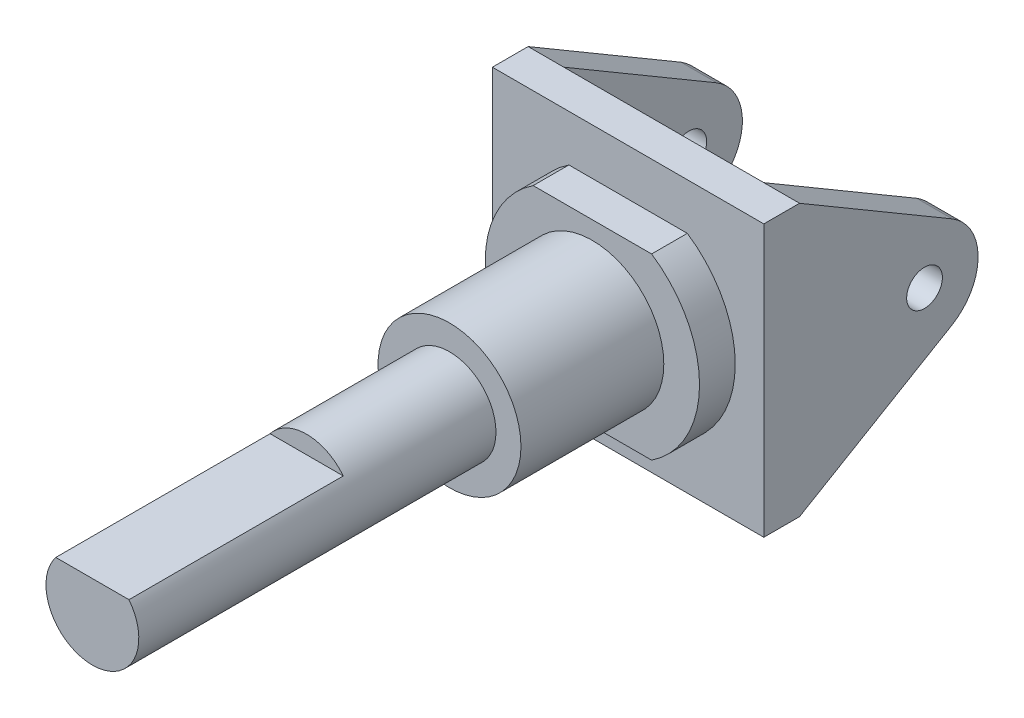
ISO-10303-21;
HEADER;
FILE_DESCRIPTION(('STEP AP214'),'2;1');
FILE_NAME('part.step','',(''),(''),'','','');
FILE_SCHEMA(('AUTOMOTIVE_DESIGN { 1 0 10303 214 1 1 1 1 }'));
ENDSEC;
DATA;
#1=APPLICATION_CONTEXT('core data for automotive mechanical design processes');
#2=APPLICATION_PROTOCOL_DEFINITION('international standard','automotive_design',2000,#1);
#3=PRODUCT_CONTEXT('',#1,'mechanical');
#4=PRODUCT('Part','Part','',(#3));
#5=PRODUCT_RELATED_PRODUCT_CATEGORY('part','',(#4));
#6=PRODUCT_DEFINITION_FORMATION('','',#4);
#7=PRODUCT_DEFINITION_CONTEXT('part definition',#1,'design');
#8=PRODUCT_DEFINITION('design','',#6,#7);
#9=PRODUCT_DEFINITION_SHAPE('','',#8);
#10=(LENGTH_UNIT() NAMED_UNIT(*) SI_UNIT(.MILLI.,.METRE.));
#11=(NAMED_UNIT(*) PLANE_ANGLE_UNIT() SI_UNIT($,.RADIAN.));
#12=(NAMED_UNIT(*) SI_UNIT($,.STERADIAN.) SOLID_ANGLE_UNIT());
#13=UNCERTAINTY_MEASURE_WITH_UNIT(LENGTH_MEASURE(1.E-05),#10,'distance_accuracy_value','');
#14=(GEOMETRIC_REPRESENTATION_CONTEXT(3) GLOBAL_UNCERTAINTY_ASSIGNED_CONTEXT((#13)) GLOBAL_UNIT_ASSIGNED_CONTEXT((#10,
#11,#12)) REPRESENTATION_CONTEXT('',''));
#15=CARTESIAN_POINT('',(0.,0.,0.));
#16=DIRECTION('',(0.,0.,1.));
#17=DIRECTION('',(1.,0.,0.));
#18=AXIS2_PLACEMENT_3D('',#15,#16,#17);
#19=CARTESIAN_POINT('',(0.,0.,20000.));
#20=DIRECTION('',(0.,0.,-1.));
#21=DIRECTION('',(-1.,0.,0.));
#22=AXIS2_PLACEMENT_3D('',#19,#20,#21);
#23=CYLINDRICAL_SURFACE('',#22,30000.);
#24=DIRECTION('',(0.,0.,-1.));
#25=VECTOR('',#24,1.);
#26=CARTESIAN_POINT('',(-16583.123951777,-25000.,20000.));
#27=LINE('',#26,#25);
#28=CARTESIAN_POINT('',(-16583.123951777,-25000.,20000.));
#29=VERTEX_POINT('',#28);
#30=CARTESIAN_POINT('',(-16583.123951777,-25000.,10000.));
#31=VERTEX_POINT('',#30);
#32=EDGE_CURVE('E194',#29,#31,#27,.T.);
#33=ORIENTED_EDGE('',*,*,#32,.F.);
#34=CARTESIAN_POINT('',(0.,0.,20000.));
#35=DIRECTION('',(0.,0.,1.));
#36=DIRECTION('',(1.,0.,0.));
#37=AXIS2_PLACEMENT_3D('',#34,#35,#36);
#38=CIRCLE('',#37,30000.);
#39=CARTESIAN_POINT('',(-16583.123951777,25000.,20000.));
#40=VERTEX_POINT('',#39);
#41=EDGE_CURVE('E197',#40,#29,#38,.T.);
#42=ORIENTED_EDGE('',*,*,#41,.F.);
#43=DIRECTION('',(0.,0.,-1.));
#44=VECTOR('',#43,1.);
#45=CARTESIAN_POINT('',(-16583.123951777,25000.,20000.));
#46=LINE('',#45,#44);
#47=CARTESIAN_POINT('',(-16583.123951777,25000.,10000.));
#48=VERTEX_POINT('',#47);
#49=EDGE_CURVE('E189',#48,#40,#46,.F.);
#50=ORIENTED_EDGE('',*,*,#49,.F.);
#51=CARTESIAN_POINT('',(0.,0.,10000.));
#52=DIRECTION('',(0.,0.,1.));
#53=DIRECTION('',(1.,0.,0.));
#54=AXIS2_PLACEMENT_3D('',#51,#52,#53);
#55=CIRCLE('',#54,30000.);
#56=EDGE_CURVE('E204',#48,#31,#55,.T.);
#57=ORIENTED_EDGE('',*,*,#56,.T.);
#58=EDGE_LOOP('',(#33,#42,#50,#57));
#59=FACE_BOUND('',#58,.T.);
#60=ADVANCED_FACE('F46',(#59),#23,.T.);
#61=DIRECTION('',(0.,0.,-1.));
#62=VECTOR('',#61,1.);
#63=CARTESIAN_POINT('',(16583.123951777,-25000.,20000.));
#64=LINE('',#63,#62);
#65=CARTESIAN_POINT('',(16583.123951777,-25000.,10000.));
#66=VERTEX_POINT('',#65);
#67=CARTESIAN_POINT('',(16583.123951777,-25000.,20000.));
#68=VERTEX_POINT('',#67);
#69=EDGE_CURVE('E68',#66,#68,#64,.F.);
#70=ORIENTED_EDGE('',*,*,#69,.F.);
#71=CARTESIAN_POINT('',(16583.123951777,25000.,10000.));
#72=VERTEX_POINT('',#71);
#73=EDGE_CURVE('E198',#66,#72,#55,.T.);
#74=ORIENTED_EDGE('',*,*,#73,.T.);
#75=DIRECTION('',(0.,0.,-1.));
#76=VECTOR('',#75,1.);
#77=CARTESIAN_POINT('',(16583.123951777,25000.,20000.));
#78=LINE('',#77,#76);
#79=CARTESIAN_POINT('',(16583.123951777,25000.,20000.));
#80=VERTEX_POINT('',#79);
#81=EDGE_CURVE('E188',#80,#72,#78,.T.);
#82=ORIENTED_EDGE('',*,*,#81,.F.);
#83=EDGE_CURVE('E193',#68,#80,#38,.T.);
#84=ORIENTED_EDGE('',*,*,#83,.F.);
#85=EDGE_LOOP('',(#70,#74,#82,#84));
#86=FACE_BOUND('',#85,.T.);
#87=ADVANCED_FACE('F304',(#86),#23,.T.);
#88=CARTESIAN_POINT('',(0.,0.,20000.));
#89=DIRECTION('',(0.,0.,1.));
#90=DIRECTION('',(1.,0.,0.));
#91=AXIS2_PLACEMENT_3D('',#88,#89,#90);
#92=PLANE('',#91);
#93=CARTESIAN_POINT('',(0.,0.,20000.));
#94=DIRECTION('',(0.,0.,1.));
#95=DIRECTION('',(1.,0.,0.));
#96=AXIS2_PLACEMENT_3D('',#93,#94,#95);
#97=CIRCLE('',#96,20000.);
#98=CARTESIAN_POINT('',(20000.,0.,20000.));
#99=VERTEX_POINT('',#98);
#100=EDGE_CURVE('E179',#99,#99,#97,.T.);
#101=ORIENTED_EDGE('',*,*,#100,.F.);
#102=EDGE_LOOP('',(#101));
#103=FACE_BOUND('',#102,.T.);
#104=ORIENTED_EDGE('',*,*,#41,.T.);
#105=DIRECTION('',(1.,0.,0.));
#106=VECTOR('',#105,1.);
#107=CARTESIAN_POINT('',(0.,-25000.,20000.));
#108=LINE('',#107,#106);
#109=EDGE_CURVE('E183',#29,#68,#108,.T.);
#110=ORIENTED_EDGE('',*,*,#109,.T.);
#111=ORIENTED_EDGE('',*,*,#83,.T.);
#112=DIRECTION('',(-1.,0.,0.));
#113=VECTOR('',#112,1.);
#114=CARTESIAN_POINT('',(0.,25000.,20000.));
#115=LINE('',#114,#113);
#116=EDGE_CURVE('E295',#80,#40,#115,.T.);
#117=ORIENTED_EDGE('',*,*,#116,.T.);
#118=EDGE_LOOP('',(#104,#110,#111,#117));
#119=FACE_BOUND('',#118,.T.);
#120=ADVANCED_FACE('F297',(#103,#119),#92,.T.);
#121=CARTESIAN_POINT('',(0.,0.,0.));
#122=DIRECTION('',(0.,0.,-1.));
#123=DIRECTION('',(-1.,0.,0.));
#124=AXIS2_PLACEMENT_3D('',#121,#122,#123);
#125=PLANE('',#124);
#126=DIRECTION('',(1.,0.,0.));
#127=VECTOR('',#126,1.);
#128=CARTESIAN_POINT('',(-38000.,-38000.,0.));
#129=LINE('',#128,#127);
#130=CARTESIAN_POINT('',(-28000.,-38000.,0.));
#131=VERTEX_POINT('',#130);
#132=CARTESIAN_POINT('',(28000.,-38000.,0.));
#133=VERTEX_POINT('',#132);
#134=EDGE_CURVE('E285',#131,#133,#129,.T.);
#135=ORIENTED_EDGE('',*,*,#134,.F.);
#136=DIRECTION('',(0.,1.,0.));
#137=VECTOR('',#136,1.);
#138=CARTESIAN_POINT('',(-28000.,38000.,0.));
#139=LINE('',#138,#137);
#140=CARTESIAN_POINT('',(-28000.,38000.,0.));
#141=VERTEX_POINT('',#140);
#142=EDGE_CURVE('E219',#131,#141,#139,.T.);
#143=ORIENTED_EDGE('',*,*,#142,.T.);
#144=DIRECTION('',(-1.,0.,0.));
#145=VECTOR('',#144,1.);
#146=CARTESIAN_POINT('',(-38000.,38000.,0.));
#147=LINE('',#146,#145);
#148=CARTESIAN_POINT('',(28000.,38000.,0.));
#149=VERTEX_POINT('',#148);
#150=EDGE_CURVE('E264',#149,#141,#147,.T.);
#151=ORIENTED_EDGE('',*,*,#150,.F.);
#152=DIRECTION('',(0.,1.,0.));
#153=VECTOR('',#152,1.);
#154=CARTESIAN_POINT('',(28000.,0.,0.));
#155=LINE('',#154,#153);
#156=EDGE_CURVE('E248',#133,#149,#155,.T.);
#157=ORIENTED_EDGE('',*,*,#156,.F.);
#158=EDGE_LOOP('',(#135,#143,#151,#157));
#159=FACE_BOUND('',#158,.T.);
#160=ADVANCED_FACE('F385',(#159),#125,.T.);
#161=CARTESIAN_POINT('',(38000.,-38000.,10000.));
#162=DIRECTION('',(-1.,0.,0.));
#163=DIRECTION('',(0.,0.,1.));
#164=AXIS2_PLACEMENT_3D('',#161,#162,#163);
#165=PLANE('',#164);
#166=DIRECTION('',(0.,0.,-1.));
#167=VECTOR('',#166,1.);
#168=CARTESIAN_POINT('',(38000.,-38000.,10000.));
#169=LINE('',#168,#167);
#170=CARTESIAN_POINT('',(38000.,-38000.,10000.));
#171=VERTEX_POINT('',#170);
#172=CARTESIAN_POINT('',(38000.,-38000.,0.));
#173=VERTEX_POINT('',#172);
#174=EDGE_CURVE('E276',#171,#173,#169,.T.);
#175=ORIENTED_EDGE('',*,*,#174,.T.);
#176=DIRECTION('',(0.,0.507188321377975,-0.861835254940172));
#177=VECTOR('',#176,1.);
#178=CARTESIAN_POINT('',(38000.,-28224.8802529961,-16610.2854977837));
#179=LINE('',#178,#177);
#180=CARTESIAN_POINT('',(38000.,-12806.4007433783,-42810.));
#181=VERTEX_POINT('',#180);
#182=EDGE_CURVE('E253',#173,#181,#179,.T.);
#183=ORIENTED_EDGE('',*,*,#182,.T.);
#184=CARTESIAN_POINT('',(38000.,0.,-35000.));
#185=DIRECTION('',(1.,0.,0.));
#186=DIRECTION('',(0.,0.,-1.));
#187=AXIS2_PLACEMENT_3D('',#184,#185,#186);
#188=CIRCLE('',#187,15000.);
#189=CARTESIAN_POINT('',(38000.,12807.4778876911,-42808.2334850018));
#190=VERTEX_POINT('',#189);
#191=EDGE_CURVE('E259',#181,#190,#188,.T.);
#192=ORIENTED_EDGE('',*,*,#191,.T.);
#193=DIRECTION('',(0.,-0.507187759813916,-0.86183558541925));
#194=VECTOR('',#193,1.);
#195=CARTESIAN_POINT('',(38000.,28224.9018992078,-16610.2734760748));
#196=LINE('',#195,#194);
#197=CARTESIAN_POINT('',(38000.,38000.,0.));
#198=VERTEX_POINT('',#197);
#199=EDGE_CURVE('E241',#198,#190,#196,.T.);
#200=ORIENTED_EDGE('',*,*,#199,.F.);
#201=DIRECTION('',(0.,0.,-1.));
#202=VECTOR('',#201,1.);
#203=CARTESIAN_POINT('',(38000.,38000.,10000.));
#204=LINE('',#203,#202);
#205=CARTESIAN_POINT('',(38000.,38000.,10000.));
#206=VERTEX_POINT('',#205);
#207=EDGE_CURVE('E202',#206,#198,#204,.T.);
#208=ORIENTED_EDGE('',*,*,#207,.F.);
#209=DIRECTION('',(0.,1.,0.));
#210=VECTOR('',#209,1.);
#211=CARTESIAN_POINT('',(38000.,-38000.,10000.));
#212=LINE('',#211,#210);
#213=EDGE_CURVE('E270',#171,#206,#212,.T.);
#214=ORIENTED_EDGE('',*,*,#213,.F.);
#215=EDGE_LOOP('',(#175,#183,#192,#200,#208,#214));
#216=FACE_BOUND('',#215,.T.);
#217=CARTESIAN_POINT('',(38000.,0.,-35000.));
#218=DIRECTION('',(1.,0.,0.));
#219=DIRECTION('',(0.,0.,-1.));
#220=AXIS2_PLACEMENT_3D('',#217,#218,#219);
#221=CIRCLE('',#220,5000.);
#222=CARTESIAN_POINT('',(38000.,0.,-40000.));
#223=VERTEX_POINT('',#222);
#224=EDGE_CURVE('E231',#223,#223,#221,.T.);
#225=ORIENTED_EDGE('',*,*,#224,.F.);
#226=EDGE_LOOP('',(#225));
#227=FACE_BOUND('',#226,.T.);
#228=ADVANCED_FACE('F48',(#216,#227),#165,.F.);
#229=CARTESIAN_POINT('',(-38000.,38000.,10000.));
#230=DIRECTION('',(0.,-1.,0.));
#231=DIRECTION('',(0.,0.,-1.));
#232=AXIS2_PLACEMENT_3D('',#229,#230,#231);
#233=PLANE('',#232);
#234=EDGE_CURVE('E278',#198,#149,#147,.T.);
#235=ORIENTED_EDGE('',*,*,#234,.T.);
#236=ORIENTED_EDGE('',*,*,#150,.T.);
#237=DIRECTION('',(-1.,0.,0.));
#238=VECTOR('',#237,1.);
#239=CARTESIAN_POINT('',(-28000.,38000.,0.));
#240=LINE('',#239,#238);
#241=CARTESIAN_POINT('',(-38000.,38000.,0.));
#242=VERTEX_POINT('',#241);
#243=EDGE_CURVE('E229',#141,#242,#240,.T.);
#244=ORIENTED_EDGE('',*,*,#243,.T.);
#245=DIRECTION('',(0.,0.,-1.));
#246=VECTOR('',#245,1.);
#247=CARTESIAN_POINT('',(-38000.,38000.,10000.));
#248=LINE('',#247,#246);
#249=CARTESIAN_POINT('',(-38000.,38000.,10000.));
#250=VERTEX_POINT('',#249);
#251=EDGE_CURVE('E286',#250,#242,#248,.T.);
#252=ORIENTED_EDGE('',*,*,#251,.F.);
#253=DIRECTION('',(-1.,0.,0.));
#254=VECTOR('',#253,1.);
#255=CARTESIAN_POINT('',(-38000.,38000.,10000.));
#256=LINE('',#255,#254);
#257=EDGE_CURVE('E275',#206,#250,#256,.T.);
#258=ORIENTED_EDGE('',*,*,#257,.F.);
#259=ORIENTED_EDGE('',*,*,#207,.T.);
#260=EDGE_LOOP('',(#235,#236,#244,#252,#258,#259));
#261=FACE_BOUND('',#260,.T.);
#262=ADVANCED_FACE('F391',(#261),#233,.F.);
#263=CARTESIAN_POINT('',(-38000.,-38000.,10000.));
#264=DIRECTION('',(1.,0.,0.));
#265=DIRECTION('',(0.,0.,-1.));
#266=AXIS2_PLACEMENT_3D('',#263,#264,#265);
#267=PLANE('',#266);
#268=ORIENTED_EDGE('',*,*,#251,.T.);
#269=DIRECTION('',(0.,-0.507198614788399,-0.861829197205994));
#270=VECTOR('',#269,1.);
#271=CARTESIAN_POINT('',(-38000.,38000.,0.));
#272=LINE('',#271,#270);
#273=CARTESIAN_POINT('',(-38000.,12788.0569282436,-42840.));
#274=VERTEX_POINT('',#273);
#275=EDGE_CURVE('E210',#242,#274,#272,.T.);
#276=ORIENTED_EDGE('',*,*,#275,.T.);
#277=CARTESIAN_POINT('',(-38000.,0.,-35000.));
#278=DIRECTION('',(-1.,0.,0.));
#279=DIRECTION('',(0.,0.,1.));
#280=AXIS2_PLACEMENT_3D('',#277,#278,#279);
#281=CIRCLE('',#280,15000.);
#282=CARTESIAN_POINT('',(-38000.,-12788.0569282436,-42840.));
#283=VERTEX_POINT('',#282);
#284=EDGE_CURVE('E228',#274,#283,#281,.T.);
#285=ORIENTED_EDGE('',*,*,#284,.T.);
#286=DIRECTION('',(0.,-0.507198614788399,0.861829197205994));
#287=VECTOR('',#286,1.);
#288=CARTESIAN_POINT('',(-38000.,-38000.,0.));
#289=LINE('',#288,#287);
#290=CARTESIAN_POINT('',(-38000.,-38000.,0.));
#291=VERTEX_POINT('',#290);
#292=EDGE_CURVE('E213',#283,#291,#289,.T.);
#293=ORIENTED_EDGE('',*,*,#292,.T.);
#294=DIRECTION('',(0.,0.,-1.));
#295=VECTOR('',#294,1.);
#296=CARTESIAN_POINT('',(-38000.,-38000.,10000.));
#297=LINE('',#296,#295);
#298=CARTESIAN_POINT('',(-38000.,-38000.,10000.));
#299=VERTEX_POINT('',#298);
#300=EDGE_CURVE('E289',#299,#291,#297,.T.);
#301=ORIENTED_EDGE('',*,*,#300,.F.);
#302=DIRECTION('',(0.,-1.,0.));
#303=VECTOR('',#302,1.);
#304=CARTESIAN_POINT('',(-38000.,-38000.,10000.));
#305=LINE('',#304,#303);
#306=EDGE_CURVE('E273',#250,#299,#305,.T.);
#307=ORIENTED_EDGE('',*,*,#306,.F.);
#308=EDGE_LOOP('',(#268,#276,#285,#293,#301,#307));
#309=FACE_BOUND('',#308,.T.);
#310=CARTESIAN_POINT('',(-38000.,0.,-35000.));
#311=DIRECTION('',(-1.,0.,0.));
#312=DIRECTION('',(0.,0.,1.));
#313=AXIS2_PLACEMENT_3D('',#310,#311,#312);
#314=CIRCLE('',#313,5000.);
#315=CARTESIAN_POINT('',(-38000.,0.,-30000.));
#316=VERTEX_POINT('',#315);
#317=EDGE_CURVE('E206',#316,#316,#314,.T.);
#318=ORIENTED_EDGE('',*,*,#317,.F.);
#319=EDGE_LOOP('',(#318));
#320=FACE_BOUND('',#319,.T.);
#321=ADVANCED_FACE('F389',(#309,#320),#267,.F.);
#322=CARTESIAN_POINT('',(-38000.,-38000.,10000.));
#323=DIRECTION('',(0.,1.,0.));
#324=DIRECTION('',(0.,0.,1.));
#325=AXIS2_PLACEMENT_3D('',#322,#323,#324);
#326=PLANE('',#325);
#327=EDGE_CURVE('E271',#291,#131,#129,.T.);
#328=ORIENTED_EDGE('',*,*,#327,.T.);
#329=ORIENTED_EDGE('',*,*,#134,.T.);
#330=DIRECTION('',(1.,0.,0.));
#331=VECTOR('',#330,1.);
#332=CARTESIAN_POINT('',(28000.,-38000.,0.));
#333=LINE('',#332,#331);
#334=EDGE_CURVE('E262',#133,#173,#333,.T.);
#335=ORIENTED_EDGE('',*,*,#334,.T.);
#336=ORIENTED_EDGE('',*,*,#174,.F.);
#337=DIRECTION('',(1.,0.,0.));
#338=VECTOR('',#337,1.);
#339=CARTESIAN_POINT('',(-38000.,-38000.,10000.));
#340=LINE('',#339,#338);
#341=EDGE_CURVE('E280',#299,#171,#340,.T.);
#342=ORIENTED_EDGE('',*,*,#341,.F.);
#343=ORIENTED_EDGE('',*,*,#300,.T.);
#344=EDGE_LOOP('',(#328,#329,#335,#336,#342,#343));
#345=FACE_BOUND('',#344,.T.);
#346=ADVANCED_FACE('F382',(#345),#326,.F.);
#347=CARTESIAN_POINT('',(0.,0.,10000.));
#348=DIRECTION('',(0.,0.,-1.));
#349=DIRECTION('',(-1.,0.,0.));
#350=AXIS2_PLACEMENT_3D('',#347,#348,#349);
#351=PLANE('',#350);
#352=ORIENTED_EDGE('',*,*,#73,.F.);
#353=DIRECTION('',(1.,0.,0.));
#354=VECTOR('',#353,1.);
#355=CARTESIAN_POINT('',(-35000.,-25000.,10000.));
#356=LINE('',#355,#354);
#357=EDGE_CURVE('E187',#31,#66,#356,.T.);
#358=ORIENTED_EDGE('',*,*,#357,.F.);
#359=ORIENTED_EDGE('',*,*,#56,.F.);
#360=DIRECTION('',(-1.,0.,0.));
#361=VECTOR('',#360,1.);
#362=CARTESIAN_POINT('',(-35000.,25000.,10000.));
#363=LINE('',#362,#361);
#364=EDGE_CURVE('E174',#72,#48,#363,.T.);
#365=ORIENTED_EDGE('',*,*,#364,.F.);
#366=EDGE_LOOP('',(#352,#358,#359,#365));
#367=FACE_BOUND('',#366,.T.);
#368=ORIENTED_EDGE('',*,*,#213,.T.);
#369=ORIENTED_EDGE('',*,*,#257,.T.);
#370=ORIENTED_EDGE('',*,*,#306,.T.);
#371=ORIENTED_EDGE('',*,*,#341,.T.);
#372=EDGE_LOOP('',(#368,#369,#370,#371));
#373=FACE_BOUND('',#372,.T.);
#374=ADVANCED_FACE('F312',(#367,#373),#351,.F.);
#375=CARTESIAN_POINT('',(28000.,-28224.8802529961,-16610.2854977837));
#376=DIRECTION('',(0.,-0.861835254940172,-0.507188321377975));
#377=DIRECTION('',(0.,0.507188321377975,-0.861835254940172));
#378=AXIS2_PLACEMENT_3D('',#375,#376,#377);
#379=PLANE('',#378);
#380=ORIENTED_EDGE('',*,*,#182,.F.);
#381=ORIENTED_EDGE('',*,*,#334,.F.);
#382=DIRECTION('',(0.,0.507188321377975,-0.861835254940172));
#383=VECTOR('',#382,1.);
#384=CARTESIAN_POINT('',(28000.,-28224.8802529961,-16610.2854977837));
#385=LINE('',#384,#383);
#386=CARTESIAN_POINT('',(28000.,-12806.4007433783,-42810.));
#387=VERTEX_POINT('',#386);
#388=EDGE_CURVE('E239',#133,#387,#385,.T.);
#389=ORIENTED_EDGE('',*,*,#388,.T.);
#390=DIRECTION('',(1.,0.,0.));
#391=VECTOR('',#390,1.);
#392=CARTESIAN_POINT('',(28000.,-12806.4007433783,-42810.));
#393=LINE('',#392,#391);
#394=EDGE_CURVE('E255',#387,#181,#393,.T.);
#395=ORIENTED_EDGE('',*,*,#394,.T.);
#396=EDGE_LOOP('',(#380,#381,#389,#395));
#397=FACE_BOUND('',#396,.T.);
#398=ADVANCED_FACE('F368',(#397),#379,.T.);
#399=CARTESIAN_POINT('',(28000.,28224.9018992078,-16610.2734760748));
#400=DIRECTION('',(0.,-0.86183558541925,0.507187759813916));
#401=DIRECTION('',(0.,-0.507187759813916,-0.86183558541925));
#402=AXIS2_PLACEMENT_3D('',#399,#400,#401);
#403=PLANE('',#402);
#404=ORIENTED_EDGE('',*,*,#199,.T.);
#405=DIRECTION('',(1.,0.,0.));
#406=VECTOR('',#405,1.);
#407=CARTESIAN_POINT('',(28000.,12807.4778876911,-42808.2334850018));
#408=LINE('',#407,#406);
#409=CARTESIAN_POINT('',(28000.,12807.4778876911,-42808.2334850018));
#410=VERTEX_POINT('',#409);
#411=EDGE_CURVE('E268',#410,#190,#408,.T.);
#412=ORIENTED_EDGE('',*,*,#411,.F.);
#413=DIRECTION('',(0.,-0.507187759813916,-0.86183558541925));
#414=VECTOR('',#413,1.);
#415=CARTESIAN_POINT('',(28000.,28224.9018992078,-16610.2734760748));
#416=LINE('',#415,#414);
#417=EDGE_CURVE('E250',#149,#410,#416,.T.);
#418=ORIENTED_EDGE('',*,*,#417,.F.);
#419=ORIENTED_EDGE('',*,*,#234,.F.);
#420=EDGE_LOOP('',(#404,#412,#418,#419));
#421=FACE_BOUND('',#420,.T.);
#422=ADVANCED_FACE('F364',(#421),#403,.F.);
#423=CARTESIAN_POINT('',(28000.,0.,-35000.));
#424=DIRECTION('',(1.,0.,0.));
#425=DIRECTION('',(0.,0.,-1.));
#426=AXIS2_PLACEMENT_3D('',#423,#424,#425);
#427=CYLINDRICAL_SURFACE('',#426,5000.);
#428=CARTESIAN_POINT('',(28000.,0.,-35000.));
#429=DIRECTION('',(1.,0.,0.));
#430=DIRECTION('',(0.,0.,-1.));
#431=AXIS2_PLACEMENT_3D('',#428,#429,#430);
#432=CIRCLE('',#431,5000.);
#433=CARTESIAN_POINT('',(28000.,0.,-40000.));
#434=VERTEX_POINT('',#433);
#435=EDGE_CURVE('E240',#434,#434,#432,.T.);
#436=ORIENTED_EDGE('',*,*,#435,.F.);
#437=EDGE_LOOP('',(#436));
#438=FACE_BOUND('',#437,.T.);
#439=ORIENTED_EDGE('',*,*,#224,.T.);
#440=EDGE_LOOP('',(#439));
#441=FACE_BOUND('',#440,.T.);
#442=ADVANCED_FACE('F370',(#438,#441),#427,.F.);
#443=CARTESIAN_POINT('',(28000.,0.,-35000.));
#444=DIRECTION('',(1.,0.,0.));
#445=DIRECTION('',(0.,0.,-1.));
#446=AXIS2_PLACEMENT_3D('',#443,#444,#445);
#447=CYLINDRICAL_SURFACE('',#446,15000.);
#448=ORIENTED_EDGE('',*,*,#191,.F.);
#449=ORIENTED_EDGE('',*,*,#394,.F.);
#450=CARTESIAN_POINT('',(28000.,0.,-35000.));
#451=DIRECTION('',(1.,0.,0.));
#452=DIRECTION('',(0.,0.,-1.));
#453=AXIS2_PLACEMENT_3D('',#450,#451,#452);
#454=CIRCLE('',#453,15000.);
#455=EDGE_CURVE('E242',#387,#410,#454,.T.);
#456=ORIENTED_EDGE('',*,*,#455,.T.);
#457=ORIENTED_EDGE('',*,*,#411,.T.);
#458=EDGE_LOOP('',(#448,#449,#456,#457));
#459=FACE_BOUND('',#458,.T.);
#460=ADVANCED_FACE('F365',(#459),#447,.T.);
#461=CARTESIAN_POINT('',(28000.,0.,0.));
#462=DIRECTION('',(1.,0.,0.));
#463=DIRECTION('',(0.,0.,-1.));
#464=AXIS2_PLACEMENT_3D('',#461,#462,#463);
#465=PLANE('',#464);
#466=ORIENTED_EDGE('',*,*,#435,.T.);
#467=EDGE_LOOP('',(#466));
#468=FACE_BOUND('',#467,.T.);
#469=ORIENTED_EDGE('',*,*,#388,.F.);
#470=ORIENTED_EDGE('',*,*,#156,.T.);
#471=ORIENTED_EDGE('',*,*,#417,.T.);
#472=ORIENTED_EDGE('',*,*,#455,.F.);
#473=EDGE_LOOP('',(#469,#470,#471,#472));
#474=FACE_BOUND('',#473,.T.);
#475=ADVANCED_FACE('F356',(#468,#474),#465,.F.);
#476=CARTESIAN_POINT('',(-28000.,38000.,0.));
#477=DIRECTION('',(0.,0.861829197205995,-0.507198614788399));
#478=DIRECTION('',(0.,0.507198614788399,0.861829197205995));
#479=AXIS2_PLACEMENT_3D('',#476,#477,#478);
#480=PLANE('',#479);
#481=ORIENTED_EDGE('',*,*,#275,.F.);
#482=ORIENTED_EDGE('',*,*,#243,.F.);
#483=DIRECTION('',(0.,-0.507198614788399,-0.861829197205994));
#484=VECTOR('',#483,1.);
#485=CARTESIAN_POINT('',(-28000.,38000.,0.));
#486=LINE('',#485,#484);
#487=CARTESIAN_POINT('',(-28000.,12788.0569282436,-42840.));
#488=VERTEX_POINT('',#487);
#489=EDGE_CURVE('E212',#141,#488,#486,.T.);
#490=ORIENTED_EDGE('',*,*,#489,.T.);
#491=DIRECTION('',(-1.,0.,0.));
#492=VECTOR('',#491,1.);
#493=CARTESIAN_POINT('',(-28000.,12788.0569282436,-42840.));
#494=LINE('',#493,#492);
#495=EDGE_CURVE('E222',#488,#274,#494,.T.);
#496=ORIENTED_EDGE('',*,*,#495,.T.);
#497=EDGE_LOOP('',(#481,#482,#490,#496));
#498=FACE_BOUND('',#497,.T.);
#499=ADVANCED_FACE('F353',(#498),#480,.T.);
#500=CARTESIAN_POINT('',(-28000.,-38000.,0.));
#501=DIRECTION('',(0.,-0.861829197205995,-0.507198614788399));
#502=DIRECTION('',(0.,0.507198614788399,-0.861829197205995));
#503=AXIS2_PLACEMENT_3D('',#500,#501,#502);
#504=PLANE('',#503);
#505=ORIENTED_EDGE('',*,*,#292,.F.);
#506=DIRECTION('',(-1.,0.,0.));
#507=VECTOR('',#506,1.);
#508=CARTESIAN_POINT('',(-28000.,-12788.0569282436,-42840.));
#509=LINE('',#508,#507);
#510=CARTESIAN_POINT('',(-28000.,-12788.0569282436,-42840.));
#511=VERTEX_POINT('',#510);
#512=EDGE_CURVE('E234',#511,#283,#509,.T.);
#513=ORIENTED_EDGE('',*,*,#512,.F.);
#514=DIRECTION('',(0.,-0.507198614788399,0.861829197205994));
#515=VECTOR('',#514,1.);
#516=CARTESIAN_POINT('',(-28000.,-38000.,0.));
#517=LINE('',#516,#515);
#518=EDGE_CURVE('E217',#511,#131,#517,.T.);
#519=ORIENTED_EDGE('',*,*,#518,.T.);
#520=ORIENTED_EDGE('',*,*,#327,.F.);
#521=EDGE_LOOP('',(#505,#513,#519,#520));
#522=FACE_BOUND('',#521,.T.);
#523=ADVANCED_FACE('F347',(#522),#504,.T.);
#524=CARTESIAN_POINT('',(-28000.,0.,-35000.));
#525=DIRECTION('',(-1.,0.,0.));
#526=DIRECTION('',(0.,0.,1.));
#527=AXIS2_PLACEMENT_3D('',#524,#525,#526);
#528=CYLINDRICAL_SURFACE('',#527,15000.);
#529=ORIENTED_EDGE('',*,*,#284,.F.);
#530=ORIENTED_EDGE('',*,*,#495,.F.);
#531=CARTESIAN_POINT('',(-28000.,0.,-35000.));
#532=DIRECTION('',(-1.,0.,0.));
#533=DIRECTION('',(0.,0.,1.));
#534=AXIS2_PLACEMENT_3D('',#531,#532,#533);
#535=CIRCLE('',#534,15000.);
#536=EDGE_CURVE('E211',#488,#511,#535,.T.);
#537=ORIENTED_EDGE('',*,*,#536,.T.);
#538=ORIENTED_EDGE('',*,*,#512,.T.);
#539=EDGE_LOOP('',(#529,#530,#537,#538));
#540=FACE_BOUND('',#539,.T.);
#541=ADVANCED_FACE('F346',(#540),#528,.T.);
#542=CARTESIAN_POINT('',(-28000.,0.,-35000.));
#543=DIRECTION('',(-1.,0.,0.));
#544=DIRECTION('',(0.,0.,1.));
#545=AXIS2_PLACEMENT_3D('',#542,#543,#544);
#546=PLANE('',#545);
#547=CARTESIAN_POINT('',(-28000.,0.,-35000.));
#548=DIRECTION('',(-1.,0.,0.));
#549=DIRECTION('',(0.,0.,1.));
#550=AXIS2_PLACEMENT_3D('',#547,#548,#549);
#551=CIRCLE('',#550,5000.);
#552=CARTESIAN_POINT('',(-28000.,0.,-30000.));
#553=VERTEX_POINT('',#552);
#554=EDGE_CURVE('E205',#553,#553,#551,.T.);
#555=ORIENTED_EDGE('',*,*,#554,.T.);
#556=EDGE_LOOP('',(#555));
#557=FACE_BOUND('',#556,.T.);
#558=ORIENTED_EDGE('',*,*,#489,.F.);
#559=ORIENTED_EDGE('',*,*,#142,.F.);
#560=ORIENTED_EDGE('',*,*,#518,.F.);
#561=ORIENTED_EDGE('',*,*,#536,.F.);
#562=EDGE_LOOP('',(#558,#559,#560,#561));
#563=FACE_BOUND('',#562,.T.);
#564=ADVANCED_FACE('F345',(#557,#563),#546,.F.);
#565=CARTESIAN_POINT('',(-28000.,0.,-35000.));
#566=DIRECTION('',(-1.,0.,0.));
#567=DIRECTION('',(0.,0.,1.));
#568=AXIS2_PLACEMENT_3D('',#565,#566,#567);
#569=CYLINDRICAL_SURFACE('',#568,5000.);
#570=ORIENTED_EDGE('',*,*,#554,.F.);
#571=EDGE_LOOP('',(#570));
#572=FACE_BOUND('',#571,.T.);
#573=ORIENTED_EDGE('',*,*,#317,.T.);
#574=EDGE_LOOP('',(#573));
#575=FACE_BOUND('',#574,.T.);
#576=ADVANCED_FACE('F329',(#572,#575),#569,.F.);
#577=CARTESIAN_POINT('',(-35000.,25000.,10000.));
#578=DIRECTION('',(0.,1.,0.));
#579=DIRECTION('',(0.,0.,1.));
#580=AXIS2_PLACEMENT_3D('',#577,#578,#579);
#581=PLANE('',#580);
#582=ORIENTED_EDGE('',*,*,#81,.T.);
#583=ORIENTED_EDGE('',*,*,#364,.T.);
#584=ORIENTED_EDGE('',*,*,#49,.T.);
#585=ORIENTED_EDGE('',*,*,#116,.F.);
#586=EDGE_LOOP('',(#582,#583,#584,#585));
#587=FACE_BOUND('',#586,.T.);
#588=ADVANCED_FACE('F307',(#587),#581,.T.);
#589=CARTESIAN_POINT('',(-35000.,-25000.,10000.));
#590=DIRECTION('',(0.,-1.,0.));
#591=DIRECTION('',(0.,0.,-1.));
#592=AXIS2_PLACEMENT_3D('',#589,#590,#591);
#593=PLANE('',#592);
#594=ORIENTED_EDGE('',*,*,#32,.T.);
#595=ORIENTED_EDGE('',*,*,#357,.T.);
#596=ORIENTED_EDGE('',*,*,#69,.T.);
#597=ORIENTED_EDGE('',*,*,#109,.F.);
#598=EDGE_LOOP('',(#594,#595,#596,#597));
#599=FACE_BOUND('',#598,.T.);
#600=ADVANCED_FACE('F319',(#599),#593,.T.);
#601=CARTESIAN_POINT('',(0.,0.,60000.));
#602=DIRECTION('',(0.,0.,-1.));
#603=DIRECTION('',(-1.,0.,0.));
#604=AXIS2_PLACEMENT_3D('',#601,#602,#603);
#605=CYLINDRICAL_SURFACE('',#604,20000.);
#606=CARTESIAN_POINT('',(0.,0.,60000.));
#607=DIRECTION('',(0.,0.,1.));
#608=DIRECTION('',(1.,0.,0.));
#609=AXIS2_PLACEMENT_3D('',#606,#607,#608);
#610=CIRCLE('',#609,20000.);
#611=CARTESIAN_POINT('',(20000.,0.,60000.));
#612=VERTEX_POINT('',#611);
#613=EDGE_CURVE('E175',#612,#612,#610,.T.);
#614=ORIENTED_EDGE('',*,*,#613,.F.);
#615=EDGE_LOOP('',(#614));
#616=FACE_BOUND('',#615,.T.);
#617=ORIENTED_EDGE('',*,*,#100,.T.);
#618=EDGE_LOOP('',(#617));
#619=FACE_BOUND('',#618,.T.);
#620=ADVANCED_FACE('F318',(#616,#619),#605,.T.);
#621=CARTESIAN_POINT('',(0.,0.,60000.));
#622=DIRECTION('',(0.,0.,1.));
#623=DIRECTION('',(1.,0.,0.));
#624=AXIS2_PLACEMENT_3D('',#621,#622,#623);
#625=PLANE('',#624);
#626=CARTESIAN_POINT('',(0.,0.,60000.));
#627=DIRECTION('',(0.,0.,1.));
#628=DIRECTION('',(1.,0.,0.));
#629=AXIS2_PLACEMENT_3D('',#626,#627,#628);
#630=CIRCLE('',#629,13000.);
#631=CARTESIAN_POINT('',(13000.,0.,60000.));
#632=VERTEX_POINT('',#631);
#633=EDGE_CURVE('E165',#632,#632,#630,.T.);
#634=ORIENTED_EDGE('',*,*,#633,.F.);
#635=EDGE_LOOP('',(#634));
#636=FACE_BOUND('',#635,.T.);
#637=ORIENTED_EDGE('',*,*,#613,.T.);
#638=EDGE_LOOP('',(#637));
#639=FACE_BOUND('',#638,.T.);
#640=ADVANCED_FACE('F330',(#636,#639),#625,.T.);
#641=CARTESIAN_POINT('',(0.,0.,160000.));
#642=DIRECTION('',(0.,0.,-1.));
#643=DIRECTION('',(-1.,0.,0.));
#644=AXIS2_PLACEMENT_3D('',#641,#642,#643);
#645=CYLINDRICAL_SURFACE('',#644,13000.);
#646=CARTESIAN_POINT('',(0.,0.,160000.));
#647=DIRECTION('',(0.,0.,1.));
#648=DIRECTION('',(1.,0.,0.));
#649=AXIS2_PLACEMENT_3D('',#646,#647,#648);
#650=CIRCLE('',#649,13000.);
#651=CARTESIAN_POINT('',(-10246.9507659596,8000.,160000.));
#652=VERTEX_POINT('',#651);
#653=CARTESIAN_POINT('',(10246.9507659596,8000.,160000.));
#654=VERTEX_POINT('',#653);
#655=EDGE_CURVE('E166',#652,#654,#650,.T.);
#656=ORIENTED_EDGE('',*,*,#655,.F.);
#657=DIRECTION('',(0.,0.,-1.));
#658=VECTOR('',#657,1.);
#659=CARTESIAN_POINT('',(-10246.9507659596,8000.,160000.));
#660=LINE('',#659,#658);
#661=CARTESIAN_POINT('',(-10246.9507659596,8000.,100000.));
#662=VERTEX_POINT('',#661);
#663=EDGE_CURVE('E62',#652,#662,#660,.T.);
#664=ORIENTED_EDGE('',*,*,#663,.T.);
#665=CARTESIAN_POINT('',(0.,0.,100000.));
#666=DIRECTION('',(0.,0.,-1.));
#667=DIRECTION('',(-1.,0.,0.));
#668=AXIS2_PLACEMENT_3D('',#665,#666,#667);
#669=CIRCLE('',#668,13000.);
#670=CARTESIAN_POINT('',(10246.9507659596,8000.,100000.));
#671=VERTEX_POINT('',#670);
#672=EDGE_CURVE('E12',#662,#671,#669,.T.);
#673=ORIENTED_EDGE('',*,*,#672,.T.);
#674=DIRECTION('',(0.,0.,-1.));
#675=VECTOR('',#674,1.);
#676=CARTESIAN_POINT('',(10246.9507659596,8000.,160000.));
#677=LINE('',#676,#675);
#678=EDGE_CURVE('E160',#671,#654,#677,.F.);
#679=ORIENTED_EDGE('',*,*,#678,.T.);
#680=EDGE_LOOP('',(#656,#664,#673,#679));
#681=FACE_BOUND('',#680,.T.);
#682=ORIENTED_EDGE('',*,*,#633,.T.);
#683=EDGE_LOOP('',(#682));
#684=FACE_BOUND('',#683,.T.);
#685=ADVANCED_FACE('F168',(#681,#684),#645,.T.);
#686=CARTESIAN_POINT('',(0.,0.,160000.));
#687=DIRECTION('',(0.,0.,1.));
#688=DIRECTION('',(1.,0.,0.));
#689=AXIS2_PLACEMENT_3D('',#686,#687,#688);
#690=PLANE('',#689);
#691=DIRECTION('',(1.,0.,0.));
#692=VECTOR('',#691,1.);
#693=CARTESIAN_POINT('',(0.,8000.,160000.));
#694=LINE('',#693,#692);
#695=EDGE_CURVE('E53',#652,#654,#694,.T.);
#696=ORIENTED_EDGE('',*,*,#695,.F.);
#697=ORIENTED_EDGE('',*,*,#655,.T.);
#698=EDGE_LOOP('',(#696,#697));
#699=FACE_BOUND('',#698,.T.);
#700=ADVANCED_FACE('F171',(#699),#690,.T.);
#701=CARTESIAN_POINT('',(0.,0.,100000.));
#702=DIRECTION('',(0.,0.,-1.));
#703=DIRECTION('',(-1.,0.,0.));
#704=AXIS2_PLACEMENT_3D('',#701,#702,#703);
#705=PLANE('',#704);
#706=DIRECTION('',(1.,0.,0.));
#707=VECTOR('',#706,1.);
#708=CARTESIAN_POINT('',(-13341.8036231336,8000.,100000.));
#709=LINE('',#708,#707);
#710=EDGE_CURVE('E169',#662,#671,#709,.T.);
#711=ORIENTED_EDGE('',*,*,#710,.T.);
#712=ORIENTED_EDGE('',*,*,#672,.F.);
#713=EDGE_LOOP('',(#711,#712));
#714=FACE_BOUND('',#713,.T.);
#715=ADVANCED_FACE('F593',(#714),#705,.F.);
#716=CARTESIAN_POINT('',(-13341.8036231336,8000.,100000.));
#717=DIRECTION('',(0.,-1.,0.));
#718=DIRECTION('',(0.,0.,-1.));
#719=AXIS2_PLACEMENT_3D('',#716,#717,#718);
#720=PLANE('',#719);
#721=ORIENTED_EDGE('',*,*,#695,.T.);
#722=ORIENTED_EDGE('',*,*,#678,.F.);
#723=ORIENTED_EDGE('',*,*,#710,.F.);
#724=ORIENTED_EDGE('',*,*,#663,.F.);
#725=EDGE_LOOP('',(#721,#722,#723,#724));
#726=FACE_BOUND('',#725,.T.);
#727=ADVANCED_FACE('F157',(#726),#720,.F.);
#728=CLOSED_SHELL('',(#60,#87,#120,#160,#228,#262,#321,#346,#374,#398,#422,#442,#460,#475,#499,
#523,#541,#564,#576,#588,#600,#620,#640,#685,#700,#715,#727));
#729=MANIFOLD_SOLID_BREP('B2',#728);
#730=ADVANCED_BREP_SHAPE_REPRESENTATION('',(#18,#729),#14);
#731=SHAPE_DEFINITION_REPRESENTATION(#9,#730);
ENDSEC;
END-ISO-10303-21;
